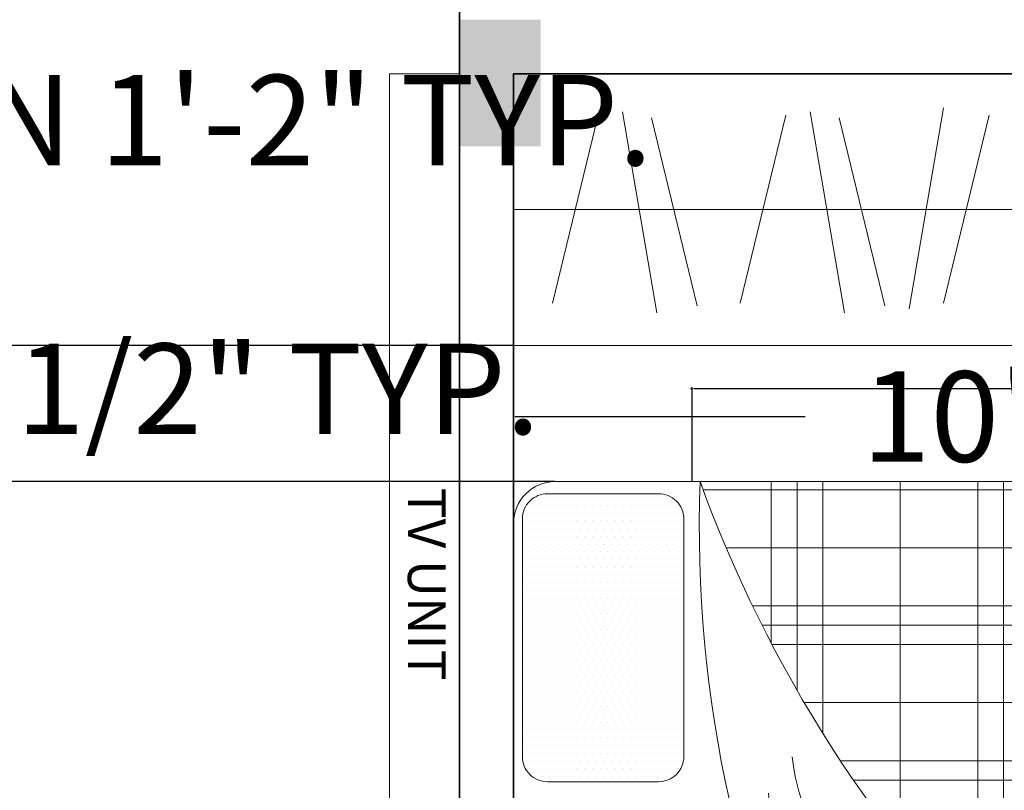
# Model space of a CAD drawing. Units: inches. Extents: x -269 to 4574, y -694 to 313.
# Tile 5 of 19: x 208 to 316, y -256 to -171. Entities that reach past the tile are written whole.
import ezdxf

# ---------------------------------------------------------------- set-up
doc = ezdxf.new("R2010")
doc.units = ezdxf.units.IN
doc.header["$MEASUREMENT"] = 0
for name, color, linetype, lineweight in [('A-COLS', 5, 'Continuous', 35), ('A-FLOR-CASE', 2, 'Continuous', 18), ('A-FURN', 2, 'Continuous', 18), ('DIMENSION', 5, 'Continuous', 18), ('TEXT', 6, 'Continuous', 18), ('WALL', 1, 'Continuous', 35)]:
    doc.layers.add(name, color=color, linetype=linetype, lineweight=lineweight)
doc.dimstyles.get("Standard").update_dxf_attribs({"dimtxt": 10, "dimasz": 0.18, "dimexe": 0.18, "dimexo": 0.0625, "dimgap": 0.09, "dimtad": 0, "dimdec": 1, "dimzin": 0, "dimdsep": 46, "dimlunit": 3, "dimtxsty": 'Standard', "dimcen": 0.09, "dimclrt": 7, "dimadec": 0, "dimazin": 0, "dimtfac": 1, "dimtdec": 1, "dimtofl": 0, "dimtmove": 0, "dimatfit": 3, "dimfxl": 1, "dimtolj": 1, "dimtzin": 0, "dimarcsym": 0})

# ---------------------------------------------------------------- blocks, each defined once
blk = doc.blocks.new('*X12')
at = {"color": 0}
for p, q in [((273.5625, 456.84375), (273.5625, 456.84375)), ((273.75, 456.9375), (273.75, 456.9375)), ((273.9375, 457.03125), (273.9375, 457.03125)), ((273.9375, 456.84375), (273.9375, 456.84375)), ((274.125, 456.9375), (274.125, 456.9375)), ((274.3125, 457.03125), (274.3125, 457.03125)), ((274.3125, 456.84375), (274.3125, 456.84375)), ((274.5, 456.9375), (274.5, 456.9375)), ((274.6875, 457.03125), (274.6875, 457.03125)), ((274.6875, 456.84375), (274.6875, 456.84375)), ((274.875, 456.9375), (274.875, 456.9375)), ((275.0625, 457.03125), (275.0625, 457.03125)), ((275.0625, 456.84375), (275.0625, 456.84375)), ((275.25, 456.9375), (275.25, 456.9375)), ((275.4375, 457.03125), (275.4375, 457.03125)), ((275.4375, 456.84375), (275.4375, 456.84375)), ((275.625, 456.9375), (275.625, 456.9375)), ((275.8125, 457.03125), (275.8125, 457.03125)), ((275.8125, 456.84375), (275.8125, 456.84375)), ((276, 456.9375), (276, 456.9375)), ((276.1875, 457.03125), (276.1875, 457.03125)), ((276.1875, 456.84375), (276.1875, 456.84375)), ((276.375, 456.9375), (276.375, 456.9375)), ((276.5625, 457.03125), (276.5625, 457.03125)), ((276.5625, 456.84375), (276.5625, 456.84375)), ((276.75, 456.9375), (276.75, 456.9375)), ((276.9375, 457.03125), (276.9375, 457.03125)), ((276.9375, 456.84375), (276.9375, 456.84375)), ((277.125, 456.9375), (277.125, 456.9375)), ((277.3125, 457.03125), (277.3125, 457.03125)), ((277.3125, 456.84375), (277.3125, 456.84375)), ((277.5, 456.9375), (277.5, 456.9375)), ((277.6875, 457.03125), (277.6875, 457.03125)), ((277.6875, 456.84375), (277.6875, 456.84375)), ((277.875, 456.9375), (277.875, 456.9375)), ((278.0625, 457.03125), (278.0625, 457.03125)), ((278.0625, 456.84375), (278.0625, 456.84375)), ((278.25, 456.9375), (278.25, 456.9375)), ((278.4375, 457.03125), (278.4375, 457.03125)), ((278.4375, 456.84375), (278.4375, 456.84375)), ((278.625, 456.9375), (278.625, 456.9375)), ((278.8125, 457.03125), (278.8125, 457.03125)), ((278.8125, 456.84375), (278.8125, 456.84375)), ((279, 456.9375), (279, 456.9375)), ((279.1875, 457.03125), (279.1875, 457.03125)), ((279.1875, 456.84375), (279.1875, 456.84375)), ((279.375, 456.9375), (279.375, 456.9375)), ((279.5625, 457.03125), (279.5625, 457.03125)), ((279.5625, 456.84375), (279.5625, 456.84375)), ((279.75, 456.9375), (279.75, 456.9375)), ((279.9375, 456.84375), (279.9375, 456.84375)), ((273.375, 456.75), (273.375, 456.75)), ((273.5625, 456.65625), (273.5625, 456.65625)), ((273.75, 456.75), (273.75, 456.75)), ((273.9375, 456.65625), (273.9375, 456.65625)), ((274.125, 456.75), (274.125, 456.75)), ((274.3125, 456.65625), (274.3125, 456.65625)), ((274.5, 456.75), (274.5, 456.75)), ((274.6875, 456.65625), (274.6875, 456.65625)), ((274.875, 456.75), (274.875, 456.75)), ((275.0625, 456.65625), (275.0625, 456.65625)), ((275.25, 456.75), (275.25, 456.75)), ((275.4375, 456.65625), (275.4375, 456.65625)), ((275.625, 456.75), (275.625, 456.75)), ((275.8125, 456.65625), (275.8125, 456.65625)), ((276, 456.75), (276, 456.75)), ((276.1875, 456.65625), (276.1875, 456.65625)), ((276.375, 456.75), (276.375, 456.75)), ((276.5625, 456.65625), (276.5625, 456.65625)), ((276.75, 456.75), (276.75, 456.75)), ((276.9375, 456.65625), (276.9375, 456.65625)), ((277.125, 456.75), (277.125, 456.75)), ((277.3125, 456.65625), (277.3125, 456.65625)), ((277.5, 456.75), (277.5, 456.75)), ((277.6875, 456.65625), (277.6875, 456.65625)), ((277.875, 456.75), (277.875, 456.75)), ((278.0625, 456.65625), (278.0625, 456.65625)), ((278.25, 456.75), (278.25, 456.75)), ((278.4375, 456.65625), (278.4375, 456.65625)), ((278.625, 456.75), (278.625, 456.75)), ((278.8125, 456.65625), (278.8125, 456.65625)), ((279, 456.75), (279, 456.75)), ((279.1875, 456.65625), (279.1875, 456.65625)), ((279.375, 456.75), (279.375, 456.75)), ((279.5625, 456.65625), (279.5625, 456.65625)), ((279.75, 456.75), (279.75, 456.75)), ((279.9375, 456.65625), (279.9375, 456.65625)), ((280.125, 456.75), (280.125, 456.75)), ((273.375, 456.5625), (273.375, 456.5625)), ((273.375, 456.375), (273.375, 456.375)), ((273.5625, 456.46875), (273.5625, 456.46875)), ((273.75, 456.5625), (273.75, 456.5625)), ((273.75, 456.375), (273.75, 456.375)), ((273.9375, 456.46875), (273.9375, 456.46875)), ((274.125, 456.5625), (274.125, 456.5625)), ((274.125, 456.375), (274.125, 456.375)), ((274.3125, 456.46875), (274.3125, 456.46875)), ((274.5, 456.5625), (274.5, 456.5625)), ((274.5, 456.375), (274.5, 456.375)), ((274.6875, 456.46875), (274.6875, 456.46875)), ((274.875, 456.5625), (274.875, 456.5625)), ((274.875, 456.375), (274.875, 456.375)), ((275.0625, 456.46875), (275.0625, 456.46875)), ((275.25, 456.5625), (275.25, 456.5625)), ((275.25, 456.375), (275.25, 456.375)), ((275.4375, 456.46875), (275.4375, 456.46875)), ((275.625, 456.5625), (275.625, 456.5625)), ((275.625, 456.375), (275.625, 456.375)), ((275.8125, 456.46875), (275.8125, 456.46875)), ((276, 456.5625), (276, 456.5625)), ((276, 456.375), (276, 456.375)), ((276.1875, 456.46875), (276.1875, 456.46875)), ((276.375, 456.5625), (276.375, 456.5625)), ((276.375, 456.375), (276.375, 456.375)), ((276.5625, 456.46875), (276.5625, 456.46875)), ((276.75, 456.5625), (276.75, 456.5625)), ((276.75, 456.375), (276.75, 456.375)), ((276.9375, 456.46875), (276.9375, 456.46875)), ((277.125, 456.5625), (277.125, 456.5625)), ((277.125, 456.375), (277.125, 456.375)), ((277.3125, 456.46875), (277.3125, 456.46875)), ((277.5, 456.5625), (277.5, 456.5625)), ((277.5, 456.375), (277.5, 456.375)), ((277.6875, 456.46875), (277.6875, 456.46875)), ((277.875, 456.5625), (277.875, 456.5625)), ((277.875, 456.375), (277.875, 456.375)), ((278.0625, 456.46875), (278.0625, 456.46875)), ((278.25, 456.5625), (278.25, 456.5625)), ((278.25, 456.375), (278.25, 456.375)), ((278.4375, 456.46875), (278.4375, 456.46875)), ((278.625, 456.5625), (278.625, 456.5625)), ((278.625, 456.375), (278.625, 456.375)), ((278.8125, 456.46875), (278.8125, 456.46875)), ((279, 456.5625), (279, 456.5625)), ((279, 456.375), (279, 456.375)), ((279.1875, 456.46875), (279.1875, 456.46875)), ((279.375, 456.5625), (279.375, 456.5625)), ((279.375, 456.375), (279.375, 456.375)), ((279.5625, 456.46875), (279.5625, 456.46875)), ((279.75, 456.5625), (279.75, 456.5625)), ((279.75, 456.375), (279.75, 456.375)), ((279.9375, 456.46875), (279.9375, 456.46875)), ((280.125, 456.5625), (280.125, 456.5625)), ((280.125, 456.375), (280.125, 456.375)), ((273.375, 456.1875), (273.375, 456.1875)), ((273.5625, 456.28125), (273.5625, 456.28125)), ((273.75, 456.1875), (273.75, 456.1875)), ((273.9375, 456.28125), (273.9375, 456.28125)), ((274.125, 456.1875), (274.125, 456.1875)), ((274.3125, 456.28125), (274.3125, 456.28125)), ((274.5, 456.1875), (274.5, 456.1875)), ((274.6875, 456.28125), (274.6875, 456.28125)), ((274.875, 456.1875), (274.875, 456.1875)), ((275.0625, 456.28125), (275.0625, 456.28125)), ((275.25, 456.1875), (275.25, 456.1875)), ((275.4375, 456.28125), (275.4375, 456.28125)), ((275.625, 456.1875), (275.625, 456.1875)), ((275.8125, 456.28125), (275.8125, 456.28125)), ((276, 456.1875), (276, 456.1875)), ((276.1875, 456.28125), (276.1875, 456.28125)), ((276.375, 456.1875), (276.375, 456.1875)), ((276.5625, 456.28125), (276.5625, 456.28125)), ((276.75, 456.1875), (276.75, 456.1875)), ((276.9375, 456.28125), (276.9375, 456.28125)), ((277.125, 456.1875), (277.125, 456.1875)), ((277.3125, 456.28125), (277.3125, 456.28125)), ((277.5, 456.1875), (277.5, 456.1875)), ((277.6875, 456.28125), (277.6875, 456.28125)), ((277.875, 456.1875), (277.875, 456.1875)), ((278.0625, 456.28125), (278.0625, 456.28125)), ((278.25, 456.1875), (278.25, 456.1875)), ((278.4375, 456.28125), (278.4375, 456.28125)), ((278.625, 456.1875), (278.625, 456.1875)), ((278.8125, 456.28125), (278.8125, 456.28125)), ((279, 456.1875), (279, 456.1875)), ((279.1875, 456.28125), (279.1875, 456.28125)), ((279.375, 456.1875), (279.375, 456.1875)), ((279.5625, 456.28125), (279.5625, 456.28125)), ((279.75, 456.1875), (279.75, 456.1875)), ((279.9375, 456.28125), (279.9375, 456.28125)), ((280.125, 456.1875), (280.125, 456.1875)), ((273.375, 456), (273.375, 456)), ((273.5625, 456.09375), (273.5625, 456.09375)), ((273.5625, 455.90625), (273.5625, 455.90625)), ((273.75, 456), (273.75, 456)), ((273.9375, 456.09375), (273.9375, 456.09375)), ((273.9375, 455.90625), (273.9375, 455.90625)), ((274.125, 456), (274.125, 456)), ((274.3125, 456.09375), (274.3125, 456.09375)), ((274.3125, 455.90625), (274.3125, 455.90625)), ((274.5, 456), (274.5, 456)), ((274.6875, 456.09375), (274.6875, 456.09375)), ((274.6875, 455.90625), (274.6875, 455.90625)), ((274.875, 456), (274.875, 456)), ((275.0625, 456.09375), (275.0625, 456.09375)), ((275.0625, 455.90625), (275.0625, 455.90625)), ((275.25, 456), (275.25, 456)), ((275.4375, 456.09375), (275.4375, 456.09375)), ((275.4375, 455.90625), (275.4375, 455.90625)), ((275.625, 456), (275.625, 456)), ((275.8125, 456.09375), (275.8125, 456.09375)), ((275.8125, 455.90625), (275.8125, 455.90625)), ((276, 456), (276, 456)), ((276.1875, 456.09375), (276.1875, 456.09375)), ((276.1875, 455.90625), (276.1875, 455.90625)), ((276.375, 456), (276.375, 456)), ((276.5625, 456.09375), (276.5625, 456.09375)), ((276.5625, 455.90625), (276.5625, 455.90625)), ((276.75, 456), (276.75, 456)), ((276.9375, 456.09375), (276.9375, 456.09375)), ((276.9375, 455.90625), (276.9375, 455.90625)), ((277.125, 456), (277.125, 456)), ((277.3125, 456.09375), (277.3125, 456.09375)), ((277.3125, 455.90625), (277.3125, 455.90625)), ((277.5, 456), (277.5, 456)), ((277.6875, 456.09375), (277.6875, 456.09375)), ((277.6875, 455.90625), (277.6875, 455.90625)), ((277.875, 456), (277.875, 456)), ((278.0625, 456.09375), (278.0625, 456.09375)), ((278.0625, 455.90625), (278.0625, 455.90625)), ((278.25, 456), (278.25, 456)), ((278.4375, 456.09375), (278.4375, 456.09375)), ((278.4375, 455.90625), (278.4375, 455.90625)), ((278.625, 456), (278.625, 456)), ((278.8125, 456.09375), (278.8125, 456.09375)), ((278.8125, 455.90625), (278.8125, 455.90625)), ((279, 456), (279, 456)), ((279.1875, 456.09375), (279.1875, 456.09375)), ((279.1875, 455.90625), (279.1875, 455.90625)), ((279.375, 456), (279.375, 456)), ((279.5625, 456.09375), (279.5625, 456.09375)), ((279.5625, 455.90625), (279.5625, 455.90625)), ((279.75, 456), (279.75, 456)), ((279.9375, 456.09375), (279.9375, 456.09375)), ((279.9375, 455.90625), (279.9375, 455.90625)), ((280.125, 456), (280.125, 456)), ((273.375, 455.8125), (273.375, 455.8125)), ((273.5625, 455.71875), (273.5625, 455.71875)), ((273.75, 455.8125), (273.75, 455.8125)), ((273.9375, 455.71875), (273.9375, 455.71875)), ((274.125, 455.8125), (274.125, 455.8125)), ((274.3125, 455.71875), (274.3125, 455.71875)), ((274.5, 455.8125), (274.5, 455.8125)), ((274.6875, 455.71875), (274.6875, 455.71875)), ((274.875, 455.8125), (274.875, 455.8125)), ((275.0625, 455.71875), (275.0625, 455.71875)), ((275.25, 455.8125), (275.25, 455.8125)), ((275.4375, 455.71875), (275.4375, 455.71875)), ((275.625, 455.8125), (275.625, 455.8125)), ((275.8125, 455.71875), (275.8125, 455.71875)), ((276, 455.8125), (276, 455.8125)), ((276.1875, 455.71875), (276.1875, 455.71875)), ((276.375, 455.8125), (276.375, 455.8125)), ((276.5625, 455.71875), (276.5625, 455.71875)), ((276.75, 455.8125), (276.75, 455.8125)), ((276.9375, 455.71875), (276.9375, 455.71875)), ((277.125, 455.8125), (277.125, 455.8125)), ((277.3125, 455.71875), (277.3125, 455.71875)), ((277.5, 455.8125), (277.5, 455.8125)), ((277.6875, 455.71875), (277.6875, 455.71875)), ((277.875, 455.8125), (277.875, 455.8125)), ((278.0625, 455.71875), (278.0625, 455.71875)), ((278.25, 455.8125), (278.25, 455.8125)), ((278.4375, 455.71875), (278.4375, 455.71875)), ((278.625, 455.8125), (278.625, 455.8125)), ((278.8125, 455.71875), (278.8125, 455.71875)), ((279, 455.8125), (279, 455.8125)), ((279.1875, 455.71875), (279.1875, 455.71875)), ((279.375, 455.8125), (279.375, 455.8125)), ((279.5625, 455.71875), (279.5625, 455.71875)), ((279.75, 455.8125), (279.75, 455.8125)), ((279.9375, 455.71875), (279.9375, 455.71875)), ((280.125, 455.8125), (280.125, 455.8125)), ((273.375, 455.625), (273.375, 455.625)), ((273.375, 455.4375), (273.375, 455.4375)), ((273.5625, 455.53125), (273.5625, 455.53125)), ((273.75, 455.625), (273.75, 455.625)), ((273.75, 455.4375), (273.75, 455.4375)), ((273.9375, 455.53125), (273.9375, 455.53125)), ((274.125, 455.625), (274.125, 455.625)), ((274.125, 455.4375), (274.125, 455.4375)), ((274.3125, 455.53125), (274.3125, 455.53125)), ((274.5, 455.625), (274.5, 455.625)), ((274.5, 455.4375), (274.5, 455.4375)), ((274.6875, 455.53125), (274.6875, 455.53125)), ((274.875, 455.625), (274.875, 455.625)), ((274.875, 455.4375), (274.875, 455.4375)), ((275.0625, 455.53125), (275.0625, 455.53125)), ((275.25, 455.625), (275.25, 455.625)), ((275.25, 455.4375), (275.25, 455.4375)), ((275.4375, 455.53125), (275.4375, 455.53125)), ((275.625, 455.625), (275.625, 455.625)), ((275.625, 455.4375), (275.625, 455.4375)), ((275.8125, 455.53125), (275.8125, 455.53125)), ((276, 455.625), (276, 455.625)), ((276, 455.4375), (276, 455.4375)), ((276.1875, 455.53125), (276.1875, 455.53125)), ((276.375, 455.625), (276.375, 455.625)), ((276.375, 455.4375), (276.375, 455.4375)), ((276.5625, 455.53125), (276.5625, 455.53125)), ((276.75, 455.625), (276.75, 455.625)), ((276.75, 455.4375), (276.75, 455.4375)), ((276.9375, 455.53125), (276.9375, 455.53125)), ((277.125, 455.625), (277.125, 455.625)), ((277.125, 455.4375), (277.125, 455.4375)), ((277.3125, 455.53125), (277.3125, 455.53125)), ((277.5, 455.625), (277.5, 455.625)), ((277.5, 455.4375), (277.5, 455.4375)), ((277.6875, 455.53125), (277.6875, 455.53125)), ((277.875, 455.625), (277.875, 455.625)), ((277.875, 455.4375), (277.875, 455.4375)), ((278.0625, 455.53125), (278.0625, 455.53125)), ((278.25, 455.625), (278.25, 455.625)), ((278.25, 455.4375), (278.25, 455.4375)), ((278.4375, 455.53125), (278.4375, 455.53125)), ((278.625, 455.625), (278.625, 455.625)), ((278.625, 455.4375), (278.625, 455.4375)), ((278.8125, 455.53125), (278.8125, 455.53125)), ((279, 455.625), (279, 455.625)), ((279, 455.4375), (279, 455.4375)), ((279.1875, 455.53125), (279.1875, 455.53125)), ((279.375, 455.625), (279.375, 455.625)), ((279.375, 455.4375), (279.375, 455.4375)), ((279.5625, 455.53125), (279.5625, 455.53125)), ((279.75, 455.625), (279.75, 455.625)), ((279.75, 455.4375), (279.75, 455.4375)), ((279.9375, 455.53125), (279.9375, 455.53125)), ((280.125, 455.625), (280.125, 455.625)), ((280.125, 455.4375), (280.125, 455.4375)), ((273.375, 455.25), (273.375, 455.25)), ((273.5625, 455.34375), (273.5625, 455.34375)), ((273.5625, 455.15625), (273.5625, 455.15625)), ((273.75, 455.25), (273.75, 455.25)), ((273.9375, 455.34375), (273.9375, 455.34375)), ((273.9375, 455.15625), (273.9375, 455.15625)), ((274.125, 455.25), (274.125, 455.25)), ((274.3125, 455.34375), (274.3125, 455.34375)), ((274.3125, 455.15625), (274.3125, 455.15625)), ((274.5, 455.25), (274.5, 455.25)), ((274.6875, 455.34375), (274.6875, 455.34375)), ((274.6875, 455.15625), (274.6875, 455.15625)), ((274.875, 455.25), (274.875, 455.25)), ((275.0625, 455.34375), (275.0625, 455.34375)), ((275.0625, 455.15625), (275.0625, 455.15625)), ((275.25, 455.25), (275.25, 455.25)), ((275.4375, 455.34375), (275.4375, 455.34375)), ((275.4375, 455.15625), (275.4375, 455.15625)), ((275.625, 455.25), (275.625, 455.25)), ((275.8125, 455.34375), (275.8125, 455.34375)), ((275.8125, 455.15625), (275.8125, 455.15625)), ((276, 455.25), (276, 455.25)), ((276.1875, 455.34375), (276.1875, 455.34375)), ((276.1875, 455.15625), (276.1875, 455.15625)), ((276.375, 455.25), (276.375, 455.25)), ((276.5625, 455.34375), (276.5625, 455.34375)), ((276.5625, 455.15625), (276.5625, 455.15625)), ((276.75, 455.25), (276.75, 455.25)), ((276.9375, 455.34375), (276.9375, 455.34375)), ((276.9375, 455.15625), (276.9375, 455.15625)), ((277.125, 455.25), (277.125, 455.25)), ((277.3125, 455.34375), (277.3125, 455.34375)), ((277.3125, 455.15625), (277.3125, 455.15625)), ((277.5, 455.25), (277.5, 455.25)), ((277.6875, 455.34375), (277.6875, 455.34375)), ((277.6875, 455.15625), (277.6875, 455.15625)), ((277.875, 455.25), (277.875, 455.25)), ((278.0625, 455.34375), (278.0625, 455.34375)), ((278.0625, 455.15625), (278.0625, 455.15625)), ((278.25, 455.25), (278.25, 455.25)), ((278.4375, 455.34375), (278.4375, 455.34375)), ((278.4375, 455.15625), (278.4375, 455.15625)), ((278.625, 455.25), (278.625, 455.25)), ((278.8125, 455.34375), (278.8125, 455.34375)), ((278.8125, 455.15625), (278.8125, 455.15625)), ((279, 455.25), (279, 455.25)), ((279.1875, 455.34375), (279.1875, 455.34375)), ((279.1875, 455.15625), (279.1875, 455.15625)), ((279.375, 455.25), (279.375, 455.25)), ((279.5625, 455.34375), (279.5625, 455.34375)), ((279.5625, 455.15625), (279.5625, 455.15625)), ((279.75, 455.25), (279.75, 455.25)), ((279.9375, 455.34375), (279.9375, 455.34375)), ((279.9375, 455.15625), (279.9375, 455.15625)), ((280.125, 455.25), (280.125, 455.25)), ((273.375, 455.0625), (273.375, 455.0625)), ((273.5625, 454.96875), (273.5625, 454.96875)), ((273.75, 455.0625), (273.75, 455.0625)), ((273.9375, 454.96875), (273.9375, 454.96875)), ((274.125, 455.0625), (274.125, 455.0625)), ((274.3125, 454.96875), (274.3125, 454.96875)), ((274.5, 455.0625), (274.5, 455.0625)), ((274.6875, 454.96875), (274.6875, 454.96875)), ((274.875, 455.0625), (274.875, 455.0625)), ((275.0625, 454.96875), (275.0625, 454.96875)), ((275.25, 455.0625), (275.25, 455.0625)), ((275.4375, 454.96875), (275.4375, 454.96875)), ((275.625, 455.0625), (275.625, 455.0625)), ((275.8125, 454.96875), (275.8125, 454.96875)), ((276, 455.0625), (276, 455.0625)), ((276.1875, 454.96875), (276.1875, 454.96875)), ((276.375, 455.0625), (276.375, 455.0625)), ((276.5625, 454.96875), (276.5625, 454.96875)), ((276.75, 455.0625), (276.75, 455.0625)), ((276.9375, 454.96875), (276.9375, 454.96875)), ((277.125, 455.0625), (277.125, 455.0625)), ((277.3125, 454.96875), (277.3125, 454.96875)), ((277.5, 455.0625), (277.5, 455.0625)), ((277.6875, 454.96875), (277.6875, 454.96875)), ((277.875, 455.0625), (277.875, 455.0625)), ((278.0625, 454.96875), (278.0625, 454.96875)), ((278.25, 455.0625), (278.25, 455.0625)), ((278.4375, 454.96875), (278.4375, 454.96875)), ((278.625, 455.0625), (278.625, 455.0625)), ((278.8125, 454.96875), (278.8125, 454.96875)), ((279, 455.0625), (279, 455.0625)), ((279.1875, 454.96875), (279.1875, 454.96875)), ((279.375, 455.0625), (279.375, 455.0625)), ((279.5625, 454.96875), (279.5625, 454.96875)), ((279.75, 455.0625), (279.75, 455.0625)), ((279.9375, 454.96875), (279.9375, 454.96875)), ((280.125, 455.0625), (280.125, 455.0625)), ((273.375, 454.875), (273.375, 454.875)), ((273.375, 454.6875), (273.375, 454.6875)), ((273.5625, 454.78125), (273.5625, 454.78125)), ((273.75, 454.875), (273.75, 454.875)), ((273.75, 454.6875), (273.75, 454.6875)), ((273.9375, 454.78125), (273.9375, 454.78125)), ((274.125, 454.875), (274.125, 454.875)), ((274.125, 454.6875), (274.125, 454.6875)), ((274.3125, 454.78125), (274.3125, 454.78125)), ((274.5, 454.875), (274.5, 454.875)), ((274.5, 454.6875), (274.5, 454.6875)), ((274.6875, 454.78125), (274.6875, 454.78125)), ((274.875, 454.875), (274.875, 454.875)), ((274.875, 454.6875), (274.875, 454.6875)), ((275.0625, 454.78125), (275.0625, 454.78125)), ((275.25, 454.875), (275.25, 454.875)), ((275.25, 454.6875), (275.25, 454.6875)), ((275.4375, 454.78125), (275.4375, 454.78125)), ((275.625, 454.875), (275.625, 454.875)), ((275.625, 454.6875), (275.625, 454.6875)), ((275.8125, 454.78125), (275.8125, 454.78125)), ((276, 454.875), (276, 454.875)), ((276, 454.6875), (276, 454.6875)), ((276.1875, 454.78125), (276.1875, 454.78125)), ((276.375, 454.875), (276.375, 454.875)), ((276.375, 454.6875), (276.375, 454.6875)), ((276.5625, 454.78125), (276.5625, 454.78125)), ((276.75, 454.875), (276.75, 454.875)), ((276.75, 454.6875), (276.75, 454.6875)), ((276.9375, 454.78125), (276.9375, 454.78125)), ((277.125, 454.875), (277.125, 454.875)), ((277.125, 454.6875), (277.125, 454.6875)), ((277.3125, 454.78125), (277.3125, 454.78125)), ((277.5, 454.875), (277.5, 454.875)), ((277.5, 454.6875), (277.5, 454.6875)), ((277.6875, 454.78125), (277.6875, 454.78125)), ((277.875, 454.875), (277.875, 454.875)), ((277.875, 454.6875), (277.875, 454.6875)), ((278.0625, 454.78125), (278.0625, 454.78125)), ((278.25, 454.875), (278.25, 454.875)), ((278.25, 454.6875), (278.25, 454.6875)), ((278.4375, 454.78125), (278.4375, 454.78125)), ((278.625, 454.875), (278.625, 454.875)), ((278.625, 454.6875), (278.625, 454.6875)), ((278.8125, 454.78125), (278.8125, 454.78125)), ((279, 454.875), (279, 454.875)), ((279, 454.6875), (279, 454.6875)), ((279.1875, 454.78125), (279.1875, 454.78125)), ((279.375, 454.875), (279.375, 454.875)), ((279.375, 454.6875), (279.375, 454.6875)), ((279.5625, 454.78125), (279.5625, 454.78125)), ((279.75, 454.875), (279.75, 454.875)), ((279.75, 454.6875), (279.75, 454.6875)), ((279.9375, 454.78125), (279.9375, 454.78125)), ((280.125, 454.875), (280.125, 454.875)), ((280.125, 454.6875), (280.125, 454.6875)), ((273.375, 454.5), (273.375, 454.5)), ((273.5625, 454.59375), (273.5625, 454.59375)), ((273.75, 454.5), (273.75, 454.5)), ((273.9375, 454.59375), (273.9375, 454.59375)), ((274.125, 454.5), (274.125, 454.5)), ((274.3125, 454.59375), (274.3125, 454.59375)), ((274.5, 454.5), (274.5, 454.5)), ((274.6875, 454.59375), (274.6875, 454.59375)), ((274.875, 454.5), (274.875, 454.5)), ((275.0625, 454.59375), (275.0625, 454.59375)), ((275.25, 454.5), (275.25, 454.5)), ((275.4375, 454.59375), (275.4375, 454.59375)), ((275.625, 454.5), (275.625, 454.5)), ((275.8125, 454.59375), (275.8125, 454.59375)), ((276, 454.5), (276, 454.5)), ((276.1875, 454.59375), (276.1875, 454.59375)), ((276.375, 454.5), (276.375, 454.5)), ((276.5625, 454.59375), (276.5625, 454.59375)), ((276.75, 454.5), (276.75, 454.5)), ((276.9375, 454.59375), (276.9375, 454.59375)), ((277.125, 454.5), (277.125, 454.5)), ((277.3125, 454.59375), (277.3125, 454.59375)), ((277.5, 454.5), (277.5, 454.5)), ((277.6875, 454.59375), (277.6875, 454.59375)), ((277.875, 454.5), (277.875, 454.5)), ((278.0625, 454.59375), (278.0625, 454.59375)), ((278.25, 454.5), (278.25, 454.5)), ((278.4375, 454.59375), (278.4375, 454.59375)), ((278.625, 454.5), (278.625, 454.5)), ((278.8125, 454.59375), (278.8125, 454.59375)), ((279, 454.5), (279, 454.5)), ((279.1875, 454.59375), (279.1875, 454.59375)), ((279.375, 454.5), (279.375, 454.5)), ((279.5625, 454.59375), (279.5625, 454.59375)), ((279.75, 454.5), (279.75, 454.5)), ((279.9375, 454.59375), (279.9375, 454.59375)), ((280.125, 454.5), (280.125, 454.5)), ((273.375, 454.3125), (273.375, 454.3125)), ((273.5625, 454.40625), (273.5625, 454.40625)), ((273.5625, 454.21875), (273.5625, 454.21875)), ((273.75, 454.3125), (273.75, 454.3125)), ((273.9375, 454.40625), (273.9375, 454.40625)), ((273.9375, 454.21875), (273.9375, 454.21875)), ((274.125, 454.3125), (274.125, 454.3125)), ((274.3125, 454.40625), (274.3125, 454.40625)), ((274.3125, 454.21875), (274.3125, 454.21875)), ((274.5, 454.3125), (274.5, 454.3125)), ((274.6875, 454.40625), (274.6875, 454.40625)), ((274.6875, 454.21875), (274.6875, 454.21875)), ((274.875, 454.3125), (274.875, 454.3125)), ((275.0625, 454.40625), (275.0625, 454.40625)), ((275.0625, 454.21875), (275.0625, 454.21875)), ((275.25, 454.3125), (275.25, 454.3125)), ((275.4375, 454.40625), (275.4375, 454.40625)), ((275.4375, 454.21875), (275.4375, 454.21875)), ((275.625, 454.3125), (275.625, 454.3125)), ((275.8125, 454.40625), (275.8125, 454.40625)), ((275.8125, 454.21875), (275.8125, 454.21875)), ((276, 454.3125), (276, 454.3125)), ((276.1875, 454.40625), (276.1875, 454.40625)), ((276.1875, 454.21875), (276.1875, 454.21875)), ((276.375, 454.3125), (276.375, 454.3125)), ((276.5625, 454.40625), (276.5625, 454.40625)), ((276.5625, 454.21875), (276.5625, 454.21875)), ((276.75, 454.3125), (276.75, 454.3125)), ((276.9375, 454.40625), (276.9375, 454.40625)), ((276.9375, 454.21875), (276.9375, 454.21875)), ((277.125, 454.3125), (277.125, 454.3125)), ((277.3125, 454.40625), (277.3125, 454.40625)), ((277.3125, 454.21875), (277.3125, 454.21875)), ((277.5, 454.3125), (277.5, 454.3125)), ((277.6875, 454.40625), (277.6875, 454.40625)), ((277.6875, 454.21875), (277.6875, 454.21875)), ((277.875, 454.3125), (277.875, 454.3125)), ((278.0625, 454.40625), (278.0625, 454.40625)), ((278.0625, 454.21875), (278.0625, 454.21875)), ((278.25, 454.3125), (278.25, 454.3125)), ((278.4375, 454.40625), (278.4375, 454.40625)), ((278.4375, 454.21875), (278.4375, 454.21875)), ((278.625, 454.3125), (278.625, 454.3125)), ((278.8125, 454.40625), (278.8125, 454.40625)), ((278.8125, 454.21875), (278.8125, 454.21875)), ((279, 454.3125), (279, 454.3125)), ((279.1875, 454.40625), (279.1875, 454.40625)), ((279.1875, 454.21875), (279.1875, 454.21875)), ((279.375, 454.3125), (279.375, 454.3125)), ((279.5625, 454.40625), (279.5625, 454.40625)), ((279.5625, 454.21875), (279.5625, 454.21875)), ((279.75, 454.3125), (279.75, 454.3125)), ((279.9375, 454.40625), (279.9375, 454.40625)), ((279.9375, 454.21875), (279.9375, 454.21875)), ((280.125, 454.3125), (280.125, 454.3125)), ((273.375, 454.125), (273.375, 454.125)), ((273.5625, 454.03125), (273.5625, 454.03125)), ((273.75, 454.125), (273.75, 454.125)), ((273.9375, 454.03125), (273.9375, 454.03125)), ((274.125, 454.125), (274.125, 454.125)), ((274.3125, 454.03125), (274.3125, 454.03125)), ((274.5, 454.125), (274.5, 454.125)), ((274.6875, 454.03125), (274.6875, 454.03125)), ((274.875, 454.125), (274.875, 454.125)), ((275.0625, 454.03125), (275.0625, 454.03125)), ((275.25, 454.125), (275.25, 454.125)), ((275.4375, 454.03125), (275.4375, 454.03125)), ((275.625, 454.125), (275.625, 454.125)), ((275.8125, 454.03125), (275.8125, 454.03125)), ((276, 454.125), (276, 454.125)), ((276.1875, 454.03125), (276.1875, 454.03125)), ((276.375, 454.125), (276.375, 454.125)), ((276.5625, 454.03125), (276.5625, 454.03125)), ((276.75, 454.125), (276.75, 454.125)), ((276.9375, 454.03125), (276.9375, 454.03125)), ((277.125, 454.125), (277.125, 454.125)), ((277.3125, 454.03125), (277.3125, 454.03125)), ((277.5, 454.125), (277.5, 454.125)), ((277.6875, 454.03125), (277.6875, 454.03125)), ((277.875, 454.125), (277.875, 454.125)), ((278.0625, 454.03125), (278.0625, 454.03125)), ((278.25, 454.125), (278.25, 454.125)), ((278.4375, 454.03125), (278.4375, 454.03125)), ((278.625, 454.125), (278.625, 454.125)), ((278.8125, 454.03125), (278.8125, 454.03125)), ((279, 454.125), (279, 454.125)), ((279.1875, 454.03125), (279.1875, 454.03125)), ((279.375, 454.125), (279.375, 454.125)), ((279.5625, 454.03125), (279.5625, 454.03125)), ((279.75, 454.125), (279.75, 454.125)), ((279.9375, 454.03125), (279.9375, 454.03125)), ((280.125, 454.125), (280.125, 454.125)), ((273.375, 453.9375), (273.375, 453.9375)), ((273.375, 453.75), (273.375, 453.75)), ((273.5625, 453.84375), (273.5625, 453.84375)), ((273.75, 453.9375), (273.75, 453.9375)), ((273.75, 453.75), (273.75, 453.75)), ((273.9375, 453.84375), (273.9375, 453.84375)), ((274.125, 453.9375), (274.125, 453.9375)), ((274.125, 453.75), (274.125, 453.75)), ((274.3125, 453.84375), (274.3125, 453.84375)), ((274.5, 453.9375), (274.5, 453.9375)), ((274.5, 453.75), (274.5, 453.75)), ((274.6875, 453.84375), (274.6875, 453.84375)), ((274.875, 453.9375), (274.875, 453.9375)), ((274.875, 453.75), (274.875, 453.75)), ((275.0625, 453.84375), (275.0625, 453.84375)), ((275.25, 453.9375), (275.25, 453.9375)), ((275.25, 453.75), (275.25, 453.75)), ((275.4375, 453.84375), (275.4375, 453.84375)), ((275.625, 453.9375), (275.625, 453.9375)), ((275.625, 453.75), (275.625, 453.75)), ((275.8125, 453.84375), (275.8125, 453.84375)), ((276, 453.9375), (276, 453.9375)), ((276, 453.75), (276, 453.75)), ((276.1875, 453.84375), (276.1875, 453.84375)), ((276.375, 453.9375), (276.375, 453.9375)), ((276.375, 453.75), (276.375, 453.75)), ((276.5625, 453.84375), (276.5625, 453.84375)), ((276.75, 453.9375), (276.75, 453.9375)), ((276.75, 453.75), (276.75, 453.75)), ((276.9375, 453.84375), (276.9375, 453.84375)), ((277.125, 453.9375), (277.125, 453.9375)), ((277.125, 453.75), (277.125, 453.75)), ((277.3125, 453.84375), (277.3125, 453.84375)), ((277.5, 453.9375), (277.5, 453.9375)), ((277.5, 453.75), (277.5, 453.75)), ((277.6875, 453.84375), (277.6875, 453.84375)), ((277.875, 453.9375), (277.875, 453.9375)), ((277.875, 453.75), (277.875, 453.75)), ((278.0625, 453.84375), (278.0625, 453.84375)), ((278.25, 453.9375), (278.25, 453.9375)), ((278.25, 453.75), (278.25, 453.75)), ((278.4375, 453.84375), (278.4375, 453.84375)), ((278.625, 453.9375), (278.625, 453.9375)), ((278.625, 453.75), (278.625, 453.75)), ((278.8125, 453.84375), (278.8125, 453.84375)), ((279, 453.9375), (279, 453.9375)), ((279, 453.75), (279, 453.75)), ((279.1875, 453.84375), (279.1875, 453.84375)), ((279.375, 453.9375), (279.375, 453.9375)), ((279.375, 453.75), (279.375, 453.75)), ((279.5625, 453.84375), (279.5625, 453.84375)), ((279.75, 453.9375), (279.75, 453.9375)), ((279.75, 453.75), (279.75, 453.75)), ((279.9375, 453.84375), (279.9375, 453.84375)), ((280.125, 453.9375), (280.125, 453.9375)), ((280.125, 453.75), (280.125, 453.75)), ((273.375, 453.5625), (273.375, 453.5625)), ((273.5625, 453.65625), (273.5625, 453.65625)), ((273.75, 453.5625), (273.75, 453.5625)), ((273.9375, 453.65625), (273.9375, 453.65625)), ((274.125, 453.5625), (274.125, 453.5625)), ((274.3125, 453.65625), (274.3125, 453.65625)), ((274.5, 453.5625), (274.5, 453.5625)), ((274.6875, 453.65625), (274.6875, 453.65625)), ((274.875, 453.5625), (274.875, 453.5625)), ((275.0625, 453.65625), (275.0625, 453.65625)), ((275.25, 453.5625), (275.25, 453.5625)), ((275.4375, 453.65625), (275.4375, 453.65625)), ((275.625, 453.5625), (275.625, 453.5625)), ((275.8125, 453.65625), (275.8125, 453.65625)), ((276, 453.5625), (276, 453.5625)), ((276.1875, 453.65625), (276.1875, 453.65625)), ((276.375, 453.5625), (276.375, 453.5625)), ((276.5625, 453.65625), (276.5625, 453.65625)), ((276.75, 453.5625), (276.75, 453.5625)), ((276.9375, 453.65625), (276.9375, 453.65625)), ((277.125, 453.5625), (277.125, 453.5625)), ((277.3125, 453.65625), (277.3125, 453.65625)), ((277.5, 453.5625), (277.5, 453.5625)), ((277.6875, 453.65625), (277.6875, 453.65625)), ((277.875, 453.5625), (277.875, 453.5625)), ((278.0625, 453.65625), (278.0625, 453.65625)), ((278.25, 453.5625), (278.25, 453.5625)), ((278.4375, 453.65625), (278.4375, 453.65625)), ((278.625, 453.5625), (278.625, 453.5625)), ((278.8125, 453.65625), (278.8125, 453.65625)), ((279, 453.5625), (279, 453.5625)), ((279.1875, 453.65625), (279.1875, 453.65625)), ((279.375, 453.5625), (279.375, 453.5625)), ((279.5625, 453.65625), (279.5625, 453.65625)), ((279.75, 453.5625), (279.75, 453.5625)), ((279.9375, 453.65625), (279.9375, 453.65625)), ((280.125, 453.5625), (280.125, 453.5625)), ((273.375, 453.375), (273.375, 453.375)), ((273.5625, 453.46875), (273.5625, 453.46875)), ((273.5625, 453.28125), (273.5625, 453.28125)), ((273.75, 453.375), (273.75, 453.375)), ((273.9375, 453.46875), (273.9375, 453.46875)), ((273.9375, 453.28125), (273.9375, 453.28125)), ((274.125, 453.375), (274.125, 453.375)), ((274.3125, 453.46875), (274.3125, 453.46875)), ((274.3125, 453.28125), (274.3125, 453.28125)), ((274.5, 453.375), (274.5, 453.375)), ((274.6875, 453.46875), (274.6875, 453.46875)), ((274.6875, 453.28125), (274.6875, 453.28125)), ((274.875, 453.375), (274.875, 453.375)), ((275.0625, 453.46875), (275.0625, 453.46875)), ((275.0625, 453.28125), (275.0625, 453.28125)), ((275.25, 453.375), (275.25, 453.375)), ((275.4375, 453.46875), (275.4375, 453.46875)), ((275.4375, 453.28125), (275.4375, 453.28125)), ((275.625, 453.375), (275.625, 453.375)), ((275.8125, 453.46875), (275.8125, 453.46875)), ((275.8125, 453.28125), (275.8125, 453.28125)), ((276, 453.375), (276, 453.375)), ((276.1875, 453.46875), (276.1875, 453.46875)), ((276.1875, 453.28125), (276.1875, 453.28125)), ((276.375, 453.375), (276.375, 453.375)), ((276.5625, 453.46875), (276.5625, 453.46875)), ((276.5625, 453.28125), (276.5625, 453.28125)), ((276.75, 453.375), (276.75, 453.375)), ((276.9375, 453.46875), (276.9375, 453.46875)), ((276.9375, 453.28125), (276.9375, 453.28125)), ((277.125, 453.375), (277.125, 453.375)), ((277.3125, 453.46875), (277.3125, 453.46875)), ((277.3125, 453.28125), (277.3125, 453.28125)), ((277.5, 453.375), (277.5, 453.375)), ((277.6875, 453.46875), (277.6875, 453.46875)), ((277.6875, 453.28125), (277.6875, 453.28125)), ((277.875, 453.375), (277.875, 453.375)), ((278.0625, 453.46875), (278.0625, 453.46875)), ((278.0625, 453.28125), (278.0625, 453.28125)), ((278.25, 453.375), (278.25, 453.375)), ((278.4375, 453.46875), (278.4375, 453.46875)), ((278.4375, 453.28125), (278.4375, 453.28125)), ((278.625, 453.375), (278.625, 453.375)), ((278.8125, 453.46875), (278.8125, 453.46875)), ((278.8125, 453.28125), (278.8125, 453.28125)), ((279, 453.375), (279, 453.375)), ((279.1875, 453.46875), (279.1875, 453.46875)), ((279.1875, 453.28125), (279.1875, 453.28125)), ((279.375, 453.375), (279.375, 453.375)), ((279.5625, 453.46875), (279.5625, 453.46875)), ((279.5625, 453.28125), (279.5625, 453.28125)), ((279.75, 453.375), (279.75, 453.375)), ((279.9375, 453.46875), (279.9375, 453.46875)), ((279.9375, 453.28125), (279.9375, 453.28125)), ((273.75, 453.1875), (273.75, 453.1875)), ((274.125, 453.1875), (274.125, 453.1875)), ((274.5, 453.1875), (274.5, 453.1875)), ((274.875, 453.1875), (274.875, 453.1875)), ((275.25, 453.1875), (275.25, 453.1875)), ((275.625, 453.1875), (275.625, 453.1875)), ((276, 453.1875), (276, 453.1875)), ((276.375, 453.1875), (276.375, 453.1875)), ((276.75, 453.1875), (276.75, 453.1875)), ((277.125, 453.1875), (277.125, 453.1875)), ((277.5, 453.1875), (277.5, 453.1875)), ((277.875, 453.1875), (277.875, 453.1875)), ((278.25, 453.1875), (278.25, 453.1875)), ((278.625, 453.1875), (278.625, 453.1875)), ((279, 453.1875), (279, 453.1875)), ((279.375, 453.1875), (279.375, 453.1875)), ((279.75, 453.1875), (279.75, 453.1875))]:
    blk.add_line(p, q, dxfattribs=at)
blk = doc.blocks.new('*D21')
at = {"layer": 'Defpoints', "color": 0, "lineweight": 0, "transparency": 16777216}
for p in [(262.14, -206.73), (388.14, -206.73), (262.14, -214.6)]:
    blk.add_point(p, dxfattribs=at)
at = {"layer": 'DIMENSION', "color": 0, "lineweight": -2, "transparency": 16777216}
for p, q in [((262.14, -206.79), (262.14, -214.78)), ((388.14, -206.79), (388.14, -214.78)), ((262.32, -214.6), (294.33, -214.6)), ((387.96, -214.6), (355.94, -214.6))]:
    blk.add_line(p, q, dxfattribs=at)
at = {"layer": 'DIMENSION', "color": 0, "lineweight": 0, "transparency": 16777216}
for points in [[(262.32, -214.57), (262.32, -214.63), (262.14, -214.6)], [(387.96, -214.57), (387.96, -214.63), (388.14, -214.6)]]:
    blk.add_solid(points, dxfattribs=at)
at = {"layer": 'DIMENSION', "color": 0, "transparency": 16777216, "insert": (325.14, -214.6), "char_height": 10, "attachment_point": 5}
blk.add_mtext('\\A1;10\'-6.0"', dxfattribs=at)
blk = doc.blocks.new('*X10')
at = {"color": 0}
for p, q in [((276.598, 451.25), (280.51, 451.25)), ((275.455, 450.625), (280.51, 450.625)), ((274.411, 450), (280.51, 450)), ((265.51, 448.125), (267.634, 448.125)), ((271.723, 448.125), (280.51, 448.125)), ((265.51, 446.25), (268.465, 446.25)), ((269.519, 446.25), (280.51, 446.25)), ((265.51, 445.625), (268.531, 445.625)), ((268.866, 445.625), (280.51, 445.625)), ((265.51, 445), (280.51, 445)), ((265.51, 443.125), (280.51, 443.125)), ((265.51, 441.25), (280.51, 441.25)), ((265.51, 440.625), (280.51, 440.625)), ((265.634, 440), (280.386, 440))]:
    blk.add_line(p, q, dxfattribs=at)
blk = doc.blocks.new('*X11')
at = {"color": 0}
for p, q in [((280.312, 439.886), (280.312, 452.896)), ((278.906, 439.482), (278.906, 452.338)), ((277.5, 439.482), (277.5, 451.702)), ((277.031, 439.482), (277.031, 451.471)), ((276.562, 439.482), (276.562, 451.231)), ((275.156, 439.482), (275.156, 450.451)), ((265.781, 439.797), (265.781, 449.511)), ((273.75, 439.482), (273.75, 449.576)), ((266.25, 439.517), (266.25, 449.296)), ((273.281, 439.482), (273.281, 449.261)), ((272.812, 439.482), (272.812, 448.934)), ((267.656, 439.482), (267.656, 448.095)), ((271.406, 439.482), (271.406, 447.876)), ((270, 439.482), (270, 446.689)), ((269.531, 439.482), (269.531, 446.262)), ((269.062, 439.482), (269.062, 445.817))]:
    blk.add_line(p, q, dxfattribs=at)
blk = doc.blocks.new('BED-DOUBLE-COVER')
for centre, radius, start, end in [((63.32, -75.96), 137.6, 87.8642, 117.4001), ((118.65, -76.93), 147.29, 109.926, 135.3977), ((36.86, 17.25), 36.85, 94.4436, 133.2788), ((41.52, 23.74), 27.87, 97.2157, 147.6656), ((-5.92, 27.4), 19.71, 357.3792, 72.5379)]:
    blk.add_arc(centre, radius, start, end)
at = {"xscale": 4.5633847399786, "yscale": 4.5633847399786, "zscale": 4.5633847399786}
for name in ['*X11', '*X10']:
    blk.add_blockref(name, (-1211.62, -2005.53), dxfattribs=at)
blk = doc.blocks.new('COLUMN-9x14-PLAN')
h = blk.add_hatch(color=256)
h.dxf.hatch_style = 1
h.paths.add_polyline_path([(9, 14), (0, 14), (0, 0), (9, 0), (9, 5)])
blk = doc.blocks.new('*D50')
at = {"layer": 'Defpoints', "color": 0, "lineweight": 0, "transparency": 16777216}
for p in [(281.85, -211.53), (281.85, -221.79), (344.28, -221.79)]:
    blk.add_point(p, dxfattribs=at)
at = {"layer": 'DIMENSION', "color": 0, "lineweight": -2, "transparency": 16777216}
for p, q in [((281.85, -211.53), (281.67, -211.53)), ((281.85, -221.73), (281.85, -211.35)), ((344.1, -211.53), (282.03, -211.53)), ((344.28, -221.73), (344.28, -211.35))]:
    blk.add_line(p, q, dxfattribs=at)
at = {"layer": 'DIMENSION', "color": 0, "lineweight": 0, "transparency": 16777216}
for points in [[(282.03, -211.5), (282.03, -211.56), (281.85, -211.53)], [(344.1, -211.5), (344.1, -211.56), (344.28, -211.53)]]:
    blk.add_solid(points, dxfattribs=at)
at = {"layer": 'DIMENSION', "color": 7, "transparency": 16777216, "insert": (222.77, -211.53), "char_height": 10, "attachment_point": 5}
blk.add_mtext('\\A1;5\'-2 1/2" TYP.', dxfattribs=at)
blk = doc.blocks.new('*D51')
at = {"layer": 'Defpoints', "color": 0, "lineweight": 0, "transparency": 16777216}
for p in [(128.14, -179.73), (142.14, -179.73), (142.14, -181.83)]:
    blk.add_point(p, dxfattribs=at)
at = {"layer": 'DIMENSION', "color": 0, "lineweight": -2, "transparency": 16777216}
for p, q in [((128.14, -179.79), (128.14, -182.01)), ((142.14, -179.79), (142.14, -182.01)), ((128.32, -181.83), (141.96, -181.83)), ((142.14, -181.83), (142.32, -181.83))]:
    blk.add_line(p, q, dxfattribs=at)
at = {"layer": 'DIMENSION', "color": 0, "lineweight": 0, "transparency": 16777216}
for points in [[(128.32, -181.8), (128.32, -181.86), (128.14, -181.83)], [(141.96, -181.8), (141.96, -181.86), (142.14, -181.83)]]:
    blk.add_solid(points, dxfattribs=at)
at = {"layer": 'DIMENSION', "color": 7, "transparency": 16777216, "insert": (216.93, -181.83), "char_height": 10, "attachment_point": 5}
blk.add_mtext('\\A1;COLUMN 1\'-2" TYP.', dxfattribs=at)
blk = doc.blocks.new('*D81')
at = {"layer": 'Defpoints', "color": 0, "lineweight": 0, "transparency": 16777216}
for p in [(-102.45, -206.73), (262.14, -206.73), (266.7, -221.79)]:
    blk.add_point(p, dxfattribs=at)
at = {"layer": 'DIMENSION', "color": 0, "lineweight": -2, "transparency": 16777216}
for p, q in [((-102.45, -206.73), (-102.45, -206.55)), ((262.07, -206.73), (-102.63, -206.73)), ((-102.45, -221.61), (-102.45, -206.91)), ((266.64, -221.79), (-102.63, -221.79))]:
    blk.add_line(p, q, dxfattribs=at)
at = {"layer": 'DIMENSION', "color": 0, "lineweight": 0, "transparency": 16777216}
for points in [[(-102.48, -206.91), (-102.42, -206.91), (-102.45, -206.73)], [(-102.48, -221.61), (-102.42, -221.61), (-102.45, -221.79)]]:
    blk.add_solid(points, dxfattribs=at)
at = {"layer": 'DIMENSION', "color": 7, "transparency": 16777216, "insert": (-102.45, -187.65), "char_height": 10, "attachment_point": 5, "rotation": 90}
blk.add_mtext('\\A1;1\'-3"', dxfattribs=at)

msp = doc.modelspace()

# ---------------------------------------------------------------- linework, layer by layer
at = {"layer": 'A-FLOR-CASE'}
for p, q in [((248.41, -176.73), (248.41, -306.73)), ((256.14, -176.73), (248.41, -176.73)), ((309.62, -180.48), (305.83, -202.71)), ((266.43, -202.06), (271.48, -181.28)), ((277.95, -203.15), (274.16, -180.92)), ((277.36, -181.57), (282.41, -202.35)), ((287.17, -202.06), (292.21, -181.28)), ((298.68, -203.15), (294.89, -180.92)), ((298.1, -181.57), (303.14, -202.35)), ((309.61, -202.06), (314.65, -181.28)), ((388.14, -191.73), (262.14, -191.73)), ((262.14, -206.73), (388.14, -206.73))]:
    msp.add_line(p, q, dxfattribs=at)
at = {"layer": 'A-FURN'}
for points in [[(344.28, -226.36), (344.28, -285.68, -0.414214), (339.71, -290.24), (266.7, -290.24, -0.414214), (262.14, -285.68), (262.14, -226.36, -0.414214), (266.7, -221.79), (339.71, -221.79, -0.414214)], [(280.93, -225.9), (280.93, -252.18, -0.414214), (278.15, -254.96), (265.88, -254.96, -0.414214), (263.1, -252.18), (263.1, -225.9, -0.414214), (265.88, -223.13), (278.15, -223.13, -0.414214)]]:
    msp.add_lwpolyline(points, format="xyb", close=True, dxfattribs=at)
at = {"layer": 'WALL'}
for p, q in [((256.14, -306.73), (256.14, -162.44)), ((262.14, -176.73), (388.14, -176.73)), ((262.14, -306.73), (262.14, -176.73))]:
    msp.add_line(p, q, dxfattribs=at)

# ---------------------------------------------------------------- block references
at = {"layer": 'A-COLS'}
msp.add_blockref('COLUMN-9x14-PLAN', (256.13, -184.73), dxfattribs=at)
at = {"layer": 'A-FURN', "rotation": 90.00000000000024}
msp.add_blockref('BED-DOUBLE-COVER', (344.28, -290.24), dxfattribs=at)
at = {"layer": 'A-FURN', "xscale": 4.5633847399786, "yscale": 4.5633847399786, "zscale": 4.5633847399786, "rotation": 90}
msp.add_blockref('*X12', (2348.75, -1501.87), dxfattribs=at)

# ---------------------------------------------------------------- texts
at = {"layer": 'TEXT'}
msp.add_text('TV UNIT', height=4.186, rotation=270, dxfattribs=at).set_placement((250.46, -222.45))

# ---------------------------------------------------------------- dimensions: what is measured, and where the dimension line sits
at = {"layer": 'DIMENSION'}
dim = msp.add_linear_dim(base=(142.14, -181.83), p1=(128.14, -179.73), p2=(142.14, -179.73), text='COLUMN <> TYP.', dimstyle='Standard', override={"dimdec": 1, "dimlfac": 1, "dimrnd": 0, "dimzin": 1, "dimdsep": 46, "dimlunit": 4, "dimfrac": 2}, dxfattribs=at)
dim.commit()
dim.dimension.update_dxf_attribs({"geometry": '*D51', "text_midpoint": (216.93, -181.83)})
dim = msp.add_linear_dim(base=(-102.45, -206.73), p1=(266.7, -221.79), p2=(262.14, -206.73), angle=90, dimstyle='Standard', override={"dimdec": 1, "dimlfac": 1, "dimrnd": 0, "dimzin": 1, "dimdsep": 46, "dimlunit": 4, "dimfrac": 2}, dxfattribs=at)
dim.commit()
dim.dimension.update_dxf_attribs({"geometry": '*D81', "text_midpoint": (-102.45, -187.65)})
dim = msp.add_linear_dim(base=(281.85, -211.53), p1=(344.28, -221.79), p2=(281.85, -221.79), angle=180, text='<> TYP.', dimstyle='Standard', override={"dimdec": 1, "dimlfac": 1, "dimrnd": 0, "dimzin": 1, "dimdsep": 46, "dimlunit": 4, "dimfrac": 2}, dxfattribs=at)
dim.commit()
dim.dimension.update_dxf_attribs({"geometry": '*D50', "text_midpoint": (222.77, -211.53)})
dim = msp.add_linear_dim(base=(262.14, -214.6), p1=(388.14, -206.73), p2=(262.14, -206.73), dimstyle='Standard', override={"dimclrd": 0, "dimclre": 0, "dimclrt": 0}, dxfattribs=at)
dim.commit()
dim.dimension.update_dxf_attribs({"geometry": '*D21', "text_midpoint": (325.14, -214.6)})

doc.saveas('drawing.dxf')
